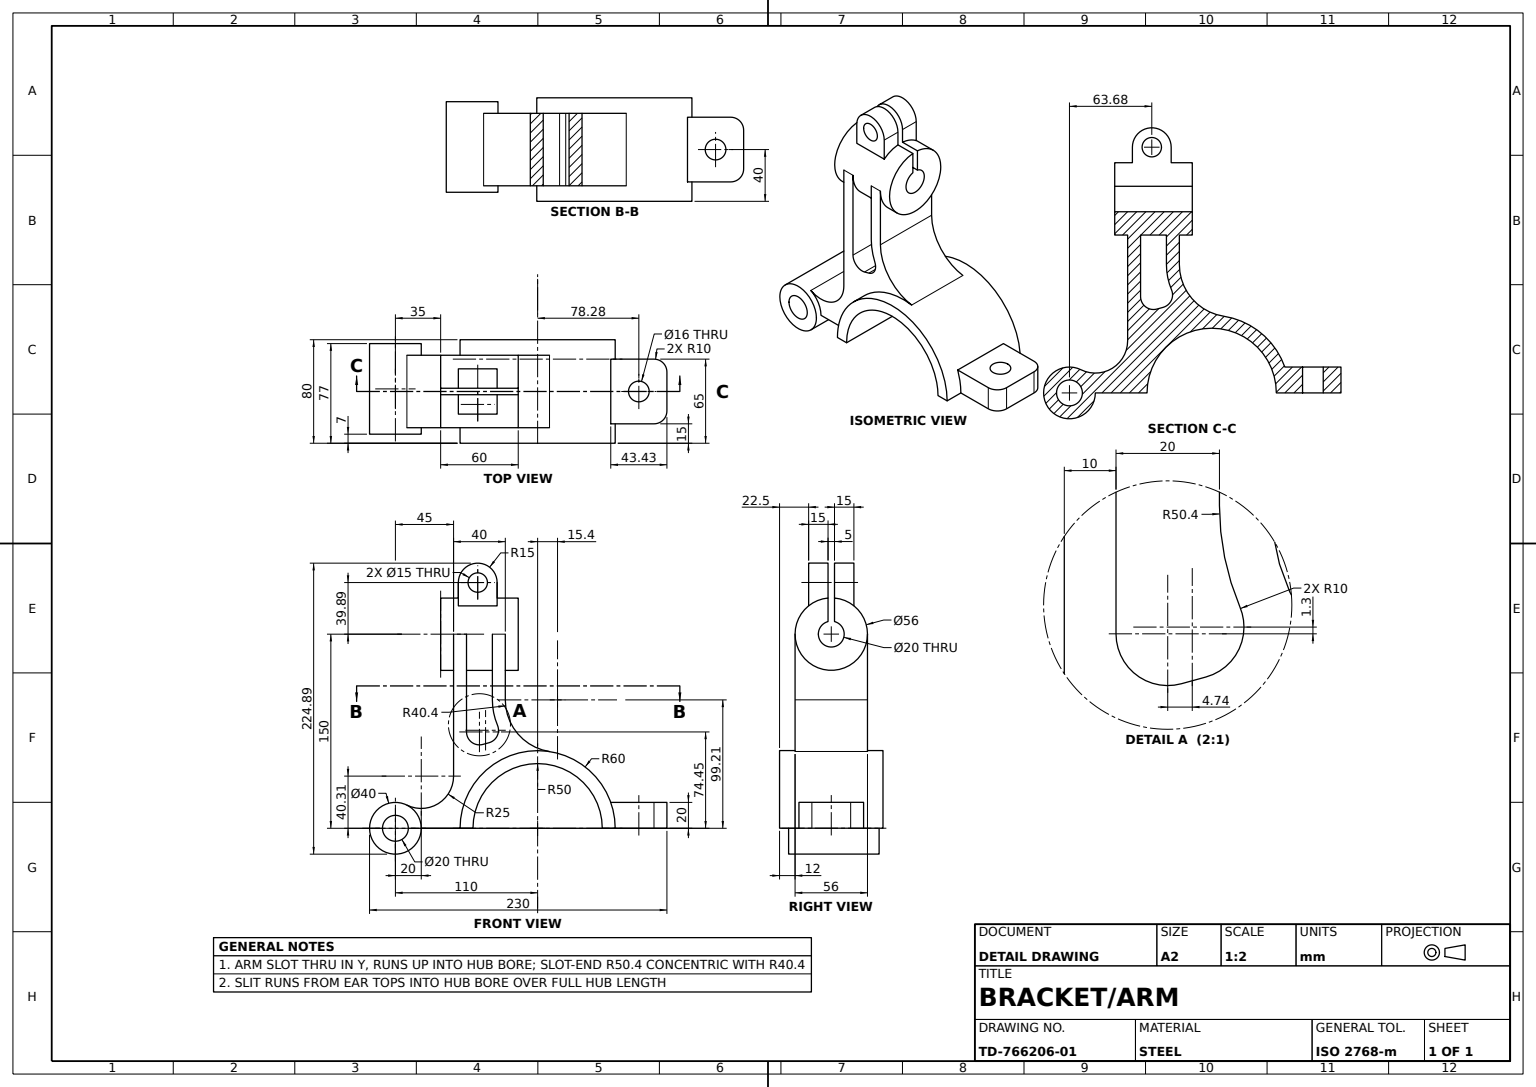
from build123d import *

# Parameters (mm, degrees)
BASE_BLOCK_DEPTH             = 40
LOWER_HUB_40_DEPTH           = 5
LOWER_HUB_40_DEPTH_BACK      = 65
LOWER_HUB_40_SKETCH_R        = 20
UPPER_HUB_56_SKETCH_R        = 28
UPPER_HUB_56_DEPTH           = 60
WEB_ARM_DEPTH                = 28
SPLIT_START                  = -101
SPLIT_SLOT_DEPTH             = 101
CLAMP_EAR_DEPTH              = 15
UPPER_BORE_20_SKETCH_R       = 10
UPPER_BORE_20_DEPTH          = 89
CLAMP_SCREW_HOLE_15_SKETCH_R = 7.5
CLAMP_SCREW_HOLE_15_DEPTH    = 89
LOWER_BORE_20_SKETCH_R       = 10
LOWER_BORE_20_DEPTH          = 89
MOUNTING_FOOT_DEPTH          = 20
FOOT_HOLE_16_SKETCH_R        = 8
FOOT_HOLE_16_DEPTH           = 45


with BuildPart() as part:
    # Base Block Sketch → Base Block (new, symmetric)
    with BuildSketch(Plane.XY):
        with BuildLine():
            Line((-60, 0), (-50, 0))
            ThreePointArc((-50, 0), (0, 50), (50, 0))
            Line((50, 0), (60, 0))
            ThreePointArc((60, 0), (0, 60), (-60, 0))
        make_face()
    extrude(amount=BASE_BLOCK_DEPTH, both=True)



with BuildPart() as body_2:
    # Lower Hub Ø40 Sketch → Lower Hub Ø40 (new, two sides: drawn at the far end of the back side and taken through both)
    with BuildSketch(Plane.XY.offset(28).offset(-LOWER_HUB_40_DEPTH_BACK)):
        with Locations((-110, 0)):
            Circle(LOWER_HUB_40_SKETCH_R)
    extrude(amount=LOWER_HUB_40_DEPTH + LOWER_HUB_40_DEPTH_BACK)


with BuildPart() as body_3:
    # Upper Hub Ø56 Sketch → Upper Hub Ø56 (new body)
    with BuildSketch(Plane(origin=(-15, 0, 0), x_dir=(0, 0, -1), z_dir=(1, 0, 0))):
        with Locations((0, 150)):
            Circle(UPPER_HUB_56_SKETCH_R)
    extrude(amount=-UPPER_HUB_56_DEPTH)


with BuildPart() as part_1:
    add(part.part)

    add(body_2.part)  # Web Arm merges body 2

    add(body_3.part)  # Web Arm merges body 3
    # Web Arm Profile → Web Arm (add, symmetric)
    with BuildSketch(Plane.XY):
        with BuildLine():
            Line((-55, 74.446056073), (-55, 150))
            Line((-55, 150), (-65, 150))
            Line((-65, 150), (-65, 40.311288741))
            ThreePointArc((-65, 40.311288741), (-76.823843083, 19.065374102), (-101.111111111, 17.91612833))
            ThreePointArc((-101.111111111, 17.91612833), (-93.003268288, 10.540925534), (-90, 0))
            Line((-90, 0), (-60, 0))
            ThreePointArc((-60, 0), (-39.037382491, 45.564051271), (9.202758941, 59.290043244))
            ThreePointArc((9.202758941, 59.290043244), (-15.279998201, 72.92654907), (-25, 99.211169164))
            Line((-25, 99.211169164), (-25, 150))
            Line((-25, 150), (-35, 150))
            Line((-35, 150), (-35, 99.211169164))
            ThreePointArc((-35, 99.211169164), (-34.000437544, 89.223422766), (-31.041398663, 79.631848749))
            ThreePointArc((-31.041398663, 79.631848749), (-31.260550889, 71.378609178), (-37.611325277, 66.103037571))
            Line((-37.611325277, 66.103037571), (-42.35537658, 64.802095944))
            ThreePointArc((-42.35537658, 64.802095944), (-51.064394685, 66.494759506), (-55, 74.446056073))
        make_face()
    extrude(amount=WEB_ARM_DEPTH, both=True)

    # Split Slot Sketch → Split Slot (cut)
    with BuildSketch(Plane.ZY.offset(75).offset(SPLIT_START)):
        with BuildLine():
            Line((-2.5, 150), (0, 150))
            Line((0, 150), (2.5, 150))
            Line((2.5, 150), (2.5, 159.682458366))
            Line((2.5, 159.682458366), (2.5, 177.888169535))
            ThreePointArc((2.5, 177.888169535), (0, 178), (-2.5, 177.888169535))
            Line((-2.5, 177.888169535), (-2.5, 159.682458366))
            Line((-2.5, 159.682458366), (-2.5, 150))
        make_face()
        with BuildLine():
            Line((2.5, 150), (0, 150))
            Line((0, 150), (-2.5, 150))
            Line((-2.5, 150), (-2.5, 159.682458366))
            ThreePointArc((-2.5, 159.682458366), (0, 140), (2.5, 159.682458366))
            Line((2.5, 159.682458366), (2.5, 150))
        make_face()
    extrude(amount=SPLIT_SLOT_DEPTH, mode=Mode.SUBTRACT)

    # Clamp Ear Sketch → Clamp Ear (add)
    with BuildSketch(Plane.XY.offset(-2.5)):
        with BuildLine():
            Line((-31.323438353, 177.888169535), (-31.323438353, 149.888169535))
            Line((-31.323438353, 149.888169535), (-61.323438353, 150))
            Line((-61.323438353, 150), (-61.323438353, 177.888169535))
            Line((-61.323438353, 177.888169535), (-61.323438353, 189.888169535))
            ThreePointArc((-61.323438353, 189.888169535), (-46.323438353, 204.888169535), (-31.323438353, 189.888169535))
            Line((-31.323438353, 189.888169535), (-31.323438353, 177.888169535))
        make_face()
    clamp_ear = extrude(amount=-CLAMP_EAR_DEPTH)

    # Clamp Ear Mirror: Clamp Ear across plane
    add(clamp_ear.mirror(Plane.XY))

    # Upper Bore Ø20 Sketch → Upper Bore Ø20 (cut)
    with BuildSketch(Plane(origin=(-15, 0, 0), x_dir=(0, 0, -1), z_dir=(1, 0, 0))):
        with Locations((0, 150)):
            Circle(UPPER_BORE_20_SKETCH_R)
    extrude(amount=-UPPER_BORE_20_DEPTH, mode=Mode.SUBTRACT)

    # Clamp Screw Hole Ø15 Sketch → Clamp Screw Hole Ø15 (cut)
    with BuildSketch(Plane.XY.offset(17.5)):
        with Locations((-46.323438353, 189.888169535)):
            Circle(CLAMP_SCREW_HOLE_15_SKETCH_R)
    extrude(amount=-CLAMP_SCREW_HOLE_15_DEPTH, mode=Mode.SUBTRACT)

    # Lower Bore Ø20 Sketch → Lower Bore Ø20 (cut)
    with BuildSketch(Plane.XY.offset(33)):
        with Locations((-110, 0)):
            Circle(LOWER_BORE_20_SKETCH_R)
    extrude(amount=-LOWER_BORE_20_DEPTH, mode=Mode.SUBTRACT)

    # Mounting Foot Sketch → Mounting Foot (add)
    with BuildSketch(Plane.XZ):
        with BuildLine():
            Line((100, 0), (100, 15))
            ThreePointArc((100, 15), (97.071067812, 22.071067812), (90, 25))
            Line((90, 25), (50, 25))
            Line((50, 25), (50, -25))
            Line((50, -25), (90, -25))
            ThreePointArc((90, -25), (97.071067812, -22.071067812), (100, -15))
            Line((100, -15), (100, 0))
        make_face()
    extrude(amount=-MOUNTING_FOOT_DEPTH)

    # Foot Hole Ø16 Sketch → Foot Hole Ø16 (cut)
    with BuildSketch(Plane(origin=(0, 20, 0), x_dir=(1, 0, 0), z_dir=(0, 1, 0))):
        with Locations(Location((78.284271247, 0, 0), (0, 0, 270))):
            Circle(FOOT_HOLE_16_SKETCH_R)
    extrude(amount=-FOOT_HOLE_16_DEPTH, mode=Mode.SUBTRACT)


solid = part_1.part
